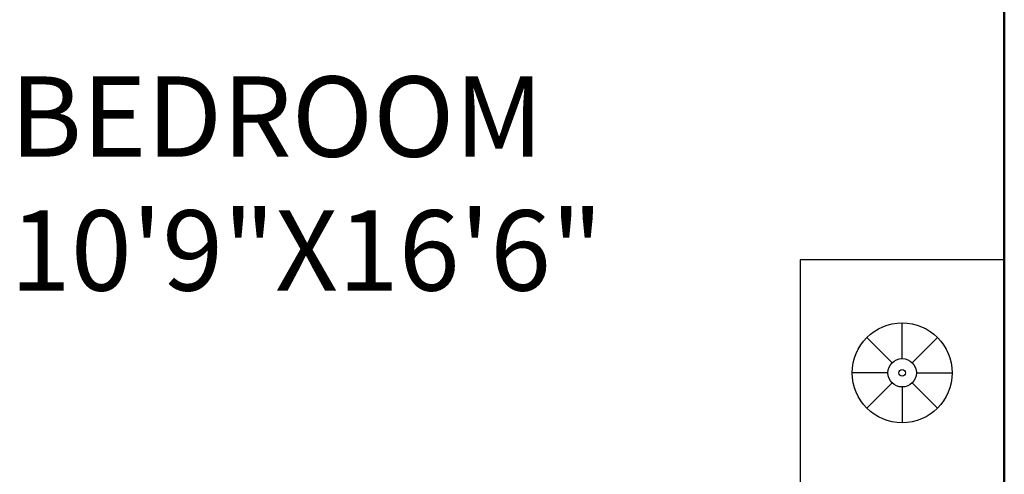
# Model space of a CAD drawing. Units: inches. Extents: x 3064 to 19385, y 846 to 15425.
# Tile 16 of 108: x 3697 to 3782, y 1094 to 1134. Entities that reach past the tile are written whole.
import ezdxf

# ---------------------------------------------------------------- set-up
doc = ezdxf.new("R2010")
doc.units = ezdxf.units.IN
for name, color, linetype, lineweight in [('A-AREA-IDEN', 3, 'Continuous', 18), ('A-FLOR-FIXT', 9, 'Continuous', 18), ('A-WALL', 7, 'Continuous', 50)]:
    doc.layers.add(name, color=color, linetype=linetype, lineweight=lineweight)
doc.layers.add('BLOCK', color=6, linetype='Continuous')
doc.styles.get("Standard").update_dxf_attribs({"font": 'arial.ttf'})

# ---------------------------------------------------------------- blocks, each defined once
blk = doc.blocks.new('A$C52E67D0D')
at = {"layer": 'BLOCK'}
for p, q in [((250.5, 1605.5), (250.5, 1684.7)), ((228.3, 1596.3), (172.3, 1652.3)), ((272.7, 1596.3), (328.7, 1652.3)), ((219.1, 1574.1), (139.9, 1574.1)), ((281.9, 1574.1), (361.1, 1574.1)), ((228.3, 1551.9), (172.3, 1495.9)), ((272.7, 1551.9), (328.7, 1495.9)), ((250.5, 1542.8), (250.5, 1463.5))]:
    blk.add_line(p, q, dxfattribs=at)
blk.add_lwpolyline([(501, 1348.6), (501, 1799.6), (0, 1799.6), (0, 1348.6)], close=True, dxfattribs=at)
for radius in [110.6, 31.4, 7.46]:
    blk.add_circle((250.5, 1574.1), radius, dxfattribs=at)

msp = doc.modelspace()

# ---------------------------------------------------------------- linework, layer by layer
at = {"layer": 'A-WALL'}
msp.add_line((3782.359, 1144.34), (3782.359, 982.34), dxfattribs=at)

# ---------------------------------------------------------------- block references
at = {"layer": 'A-FLOR-FIXT', "xscale": 0.039370099999992, "yscale": 0.039370099999992, "zscale": 0.039370099999992, "rotation": 270}
msp.add_blockref('A$C52E67D0D', (3711.493, 1112.592), dxfattribs=at)

# ---------------------------------------------------------------- texts
at = {"layer": 'A-AREA-IDEN', "insert": (3695.772, 1128.57), "char_height": 7, "attachment_point": 1}
msp.add_mtext_dynamic_manual_height_columns('BEDROOM\\P10\'9"X16\'6"', width=67.59241, gutter_width=12.5, heights=[0], dxfattribs=at)

doc.saveas('drawing.dxf')
